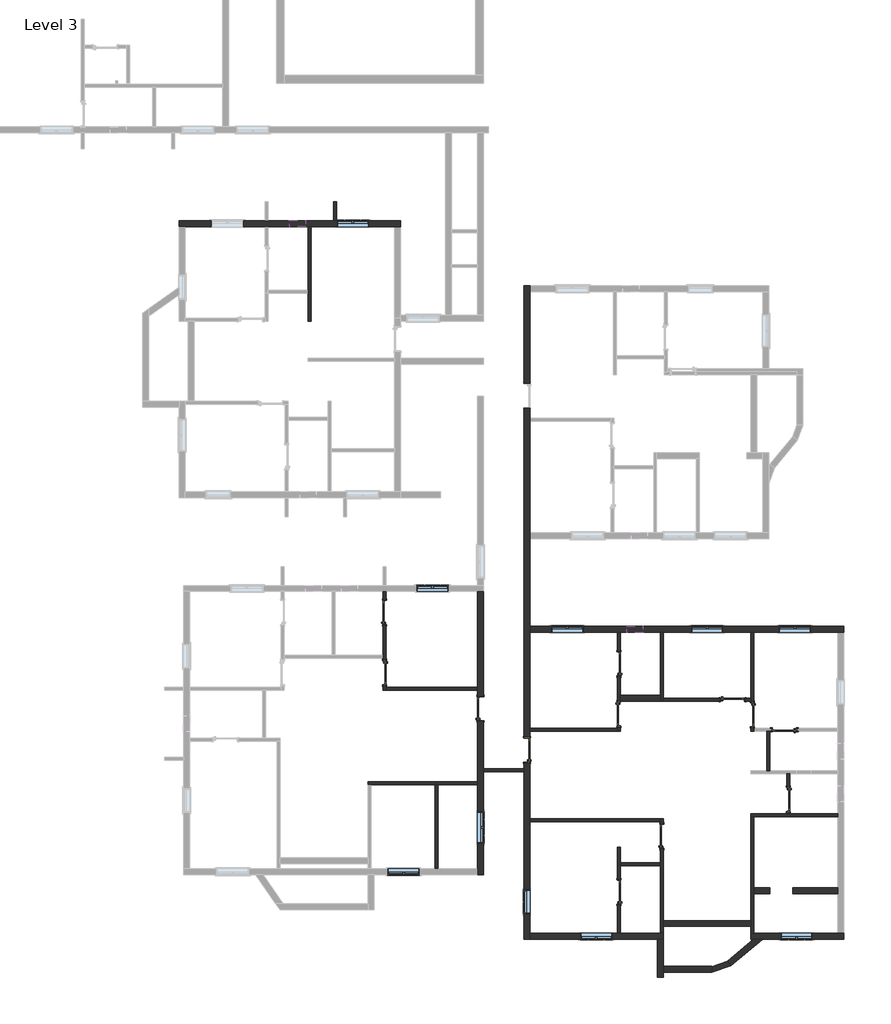
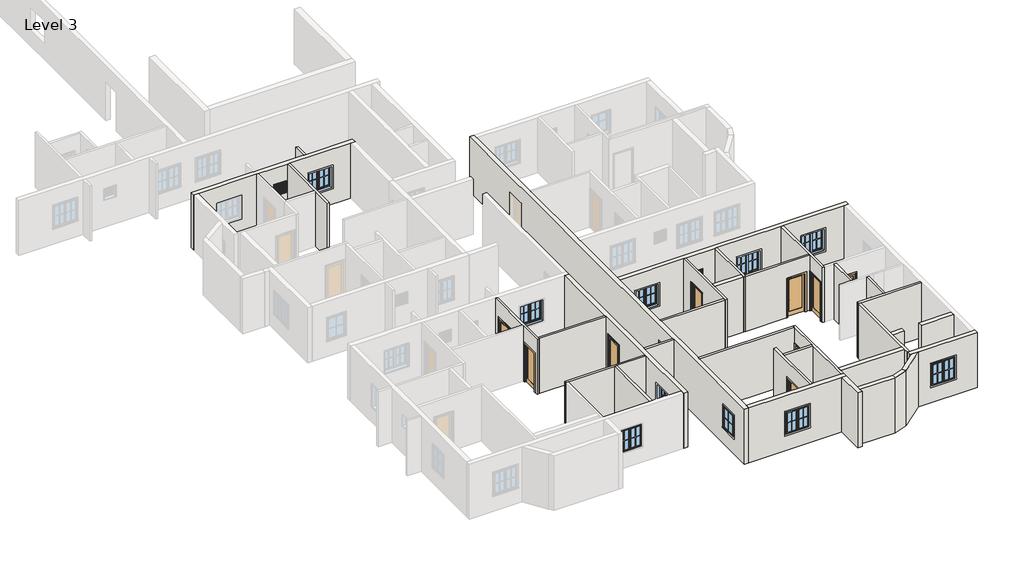
# One storey, part 2 of 7: 34 walls, 12 doors, 12 windows.
# Revit data of these elements (continued)
# Element 48 (IfcWindow, "Window-Casement-Double : 4' x 4'") (continued)
#   Materials on its faces: "Wood - Stained", "Glass", "Clad - White"
# Element 49 (IfcWindow, "Window-Casement-Double : 4' x 4'")
#   Mark = "46"
#   Window Inset = 0' - 0"
#   Interior Wall Closure = 0' - 2 1/4"
#   Frame Extension = 0' - 0 1/4"
#   Exterior Wall Closure = 0' - 1 1/4"
#   Interior Trim Visibility = yes
#   Exterior Trim Visibility = yes
#   Phase Created = New Construction
#   Materials on its faces: "Wood - Stained", "Glass", "Clad - White"
# Element 50 (IfcWindow, "Window-Casement-Double : 4' x 4'")
#   Mark = "47"
#   Window Inset = 0' - 0"
#   Interior Wall Closure = 0' - 2 1/4"
#   Frame Extension = 0' - 0 1/4"
#   Exterior Wall Closure = 0' - 1 1/4"
#   Interior Trim Visibility = yes
#   Exterior Trim Visibility = yes
#   Phase Created = New Construction
#   Materials on its faces: "Wood - Stained", "Glass", "Clad - White"
# Element 51 (IfcWindow, "Window-Casement-Double : 4' x 4'")
#   Mark = "48"
#   Window Inset = 0' - 0"
#   Interior Wall Closure = 0' - 2 1/4"
#   Frame Extension = 0' - 0 1/4"
#   Exterior Wall Closure = 0' - 1 1/4"
#   Interior Trim Visibility = yes
#   Exterior Trim Visibility = yes
#   Phase Created = New Construction
#   Materials on its faces: "Wood - Stained", "Glass", "Clad - White"
# Element 52 (IfcWindow, "Window-Casement-Double : 4' x 4'")
#   Mark = "49"
#   Window Inset = 0' - 0"
#   Interior Wall Closure = 0' - 2 1/4"
#   Frame Extension = 0' - 0 1/4"
#   Exterior Wall Closure = 0' - 1 1/4"
#   Interior Trim Visibility = yes
#   Exterior Trim Visibility = yes
#   Phase Created = New Construction
#   Materials on its faces: "Wood - Stained", "Glass", "Clad - White"
# Element 53 (IfcWindow, "Window-Casement-Double : 4' x 4'")
#   Mark = "50"
#   Window Inset = 0' - 0"
#   Interior Wall Closure = 0' - 2 1/4"
#   Frame Extension = 0' - 0 1/4"
#   Exterior Wall Closure = 0' - 1 1/4"
#   Interior Trim Visibility = yes
#   Exterior Trim Visibility = yes
#   Phase Created = New Construction
#   Materials on its faces: "Wood - Stained", "Glass", "Clad - White"
# Element 54 (IfcWindow, "Window-Casement-Double : 4' x 4'")
#   Mark = "51"
#   Window Inset = 0' - 0"
#   Interior Wall Closure = 0' - 2 1/4"
#   Frame Extension = 0' - 0 1/4"
#   Exterior Wall Closure = 0' - 1 1/4"
#   Interior Trim Visibility = yes
#   Exterior Trim Visibility = yes
#   Phase Created = New Construction
#   Materials on its faces: "Wood - Stained", "Glass", "Clad - White"
# Element 55 (IfcWindow, "Window-Casement-Double : 4' x 4'")
#   Mark = "53"
#   Window Inset = 0' - 0"
#   Interior Wall Closure = 0' - 2 1/4"
#   Frame Extension = 0' - 0 1/4"
#   Exterior Wall Closure = 0' - 1 1/4"
#   Interior Trim Visibility = yes
#   Exterior Trim Visibility = yes
#   Phase Created = New Construction
#   Materials on its faces: "Wood - Stained", "Glass", "Clad - White"
# Element 56 (IfcWindow, "Window-Casement-Double : 4' x 4'")
#   Mark = "60"
#   Window Inset = 0' - 0"
#   Interior Wall Closure = 0' - 2 1/4"
#   Frame Extension = 0' - 0 1/4"
#   Exterior Wall Closure = 0' - 1 1/4"
#   Interior Trim Visibility = yes
#   Exterior Trim Visibility = yes
#   Phase Created = New Construction
#   Materials on its faces: "Wood - Stained", "Glass", "Clad - White"
# Element 57 (IfcWindow, "Window-Louvers : 24\" x 24\"")
#   Mark = "7"
#   Blade Width = 1' - 10 1/2"
#   Phase Created = New Construction
#   Materials on its faces: "Birch"
# Element 58 (IfcWindow, "Window-Louvers : 24\" x 24\"")
#   Mark = "13"
#   Blade Width = 1' - 10 1/2"
#   Phase Created = New Construction
#   Materials on its faces: "Birch"
# Materials
#   "Cherry": class "Wood", colour RGB 226 177 128, transparency 0, Description = "Prunus Serotina", Cost = 0
#   "Aluminum": class "Metal", colour RGB 247 247 247, transparency 0, Description = "Aluminum 6061", Cost = 0
#   "Wood - Stained": class "Wood", colour RGB 224 178 126, transparency 0, Cost = 0
#   "Glass": class "Glass", colour RGB 0 128 192, transparency 0.75, Description = "Soda Lime Glass", Cost = 0
#   "Clad - White": class "Wood", colour RGB 242 242 238, transparency 0, Cost = 0
#   "Birch": class "Wood", colour RGB 224 178 126, transparency 0, Description = "Betula Alleghaniensis", Cost = 0
#   "Default Wall": colour RGB 128 128 128, transparency 0, Cost = 0
